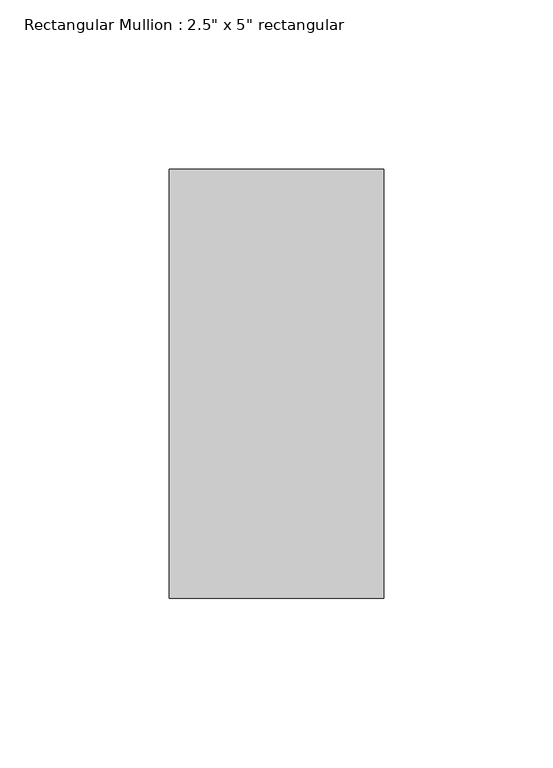
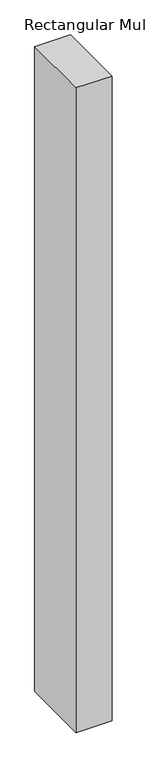
"""IFC4 building model written with IfcOpenShell, lengths in millimetres: member geometry."""

from ifc_helpers import new_model, si_unit, frame, origin, place, context, project, spatial, polyline, outline, extrude, source, transform, mapped, element, save


def member_abd5b11f(model_context):
    return source(origin(), model_context, "Body", "SweptSolid", [
        extrude(outline(polyline([(31.75, 63.5), (31.75, -63.5), (-31.75, -63.5), (-31.75, 63.5), (31.75, 63.5)])), frame((0.0, 0.0, -1206.4999998), z_axis=(0.0, 0.0, 1.0), x_axis=(1.0, 0.0, 0.0)), (0.0, 0.0, 1.0), 1206.4999998),
    ])


if __name__ == "__main__":
    model = new_model("IFC4")
    model_context = context("Model", 3, world=origin())
    ifc_project = project(units=[si_unit("LENGTHUNIT", "METRE", prefix="MILLI")], contexts=[model_context])
    site = spatial("IfcSite", under=ifc_project)
    building = spatial("IfcBuilding", under=site)
    placement = place(None, origin())
    member_shape = member_abd5b11f(model_context)
    element("IfcMember", 1, ObjectType="Rectangular Mullion : 2.5\" x 5\" rectangular", at=placement, inside=building, context=model_context, shape_type="MappedRepresentation", body=[
        mapped(member_shape, transform((0.0, 0.0, 0.0), x_axis=(1.0, 0.0, 0.0), y_axis=(0.0, 1.0, 0.0), z_axis=(0.0, 0.0, 1.0))),
    ])
    save(model, "model.ifc")

# Revit data of these elements
# Type "Rectangular Mullion : 2.5\" x 5\" rectangular"
#   built-in parameter 1007304 = 0.416667 (stored number, unit not read)
#   built-in parameter 1007301 = 0.104167 (stored number, unit not read)
#   built-in parameter 1007300 = 0.104167 (stored number, unit not read)
# Element 1 (IfcMember, "Rectangular Mullion : 2.5\" x 5\" rectangular")
#   Materials on its faces: "WINDOW FRAMING"
# Materials
#   "WINDOW FRAMING": class "Generic", colour RGB 120 120 120, transparency 0, Cost = 0
